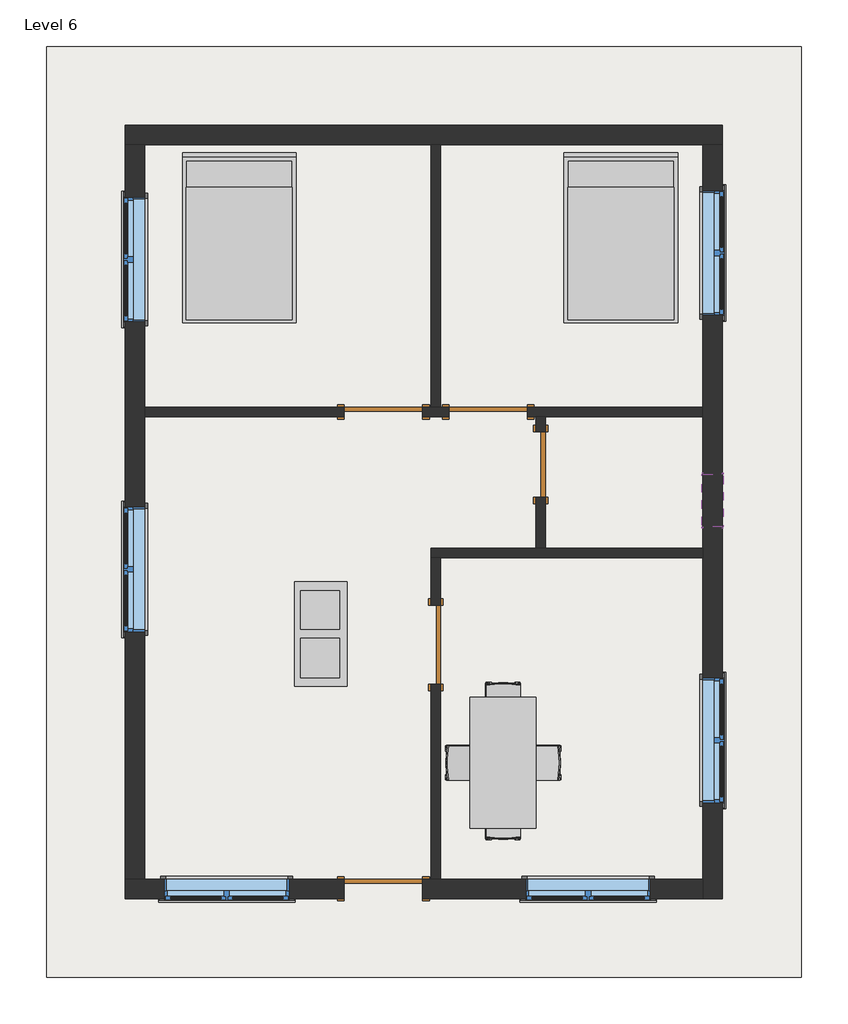
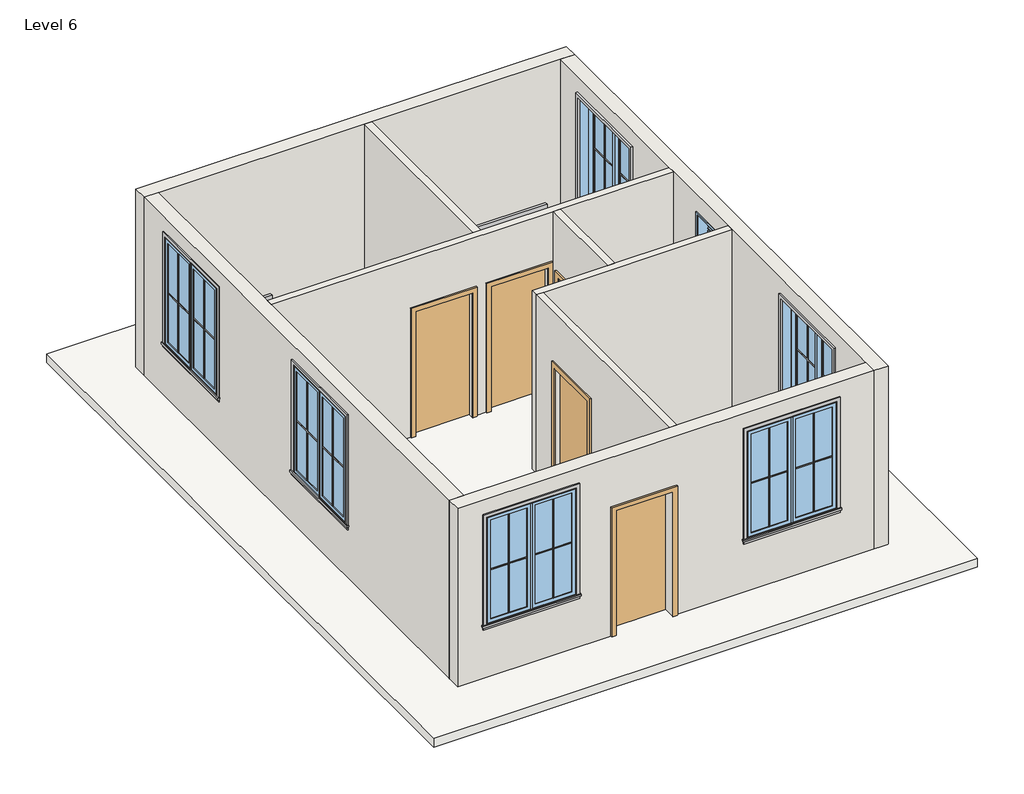
# One storey, incomplete: 25 proxies, 9 walls, 7 windows, 5 doors, 3 furniture elements, 1 roof.
"""IFC4 building model written with IfcOpenShell, lengths in millimetres."""

from ifc_helpers import new_model, si_unit, frame, origin, place, context, project, spatial, polyline, outline, extrude, faceted_brep, transform, mapped, element, save
from components import muntin_pattern_2x2_muntin_pattern_2x2_bff912c5, muntin_pattern_2x2_muntin_pattern_2x2_c2194282, trim_window_exterior_flat_with_sill_e04b3088, trim_window_interior_flat_picture_frame_2a7685fe, coffee_table_with_brass_mullions_11320_coffee_table_with_5962bef7, door_305aa2a5, door_e5f9f3c4, door_0ca8825f, door_f2b275c1, bed_17739_bed_17739_15c61121, dining_table_w_chairs_11374_0cdfc61b, window_9ac97e1a, window_f2d8fef0

model = new_model("IFC4")

# Units and contexts
model_context = context("Model", 3, world=origin())
ifc_project = project(units=[si_unit("LENGTHUNIT", "METRE", prefix="MILLI")], contexts=[model_context])

# Site, building, storey
site = spatial("IfcSite", under=ifc_project)
building = spatial("IfcBuilding", under=site)
storey = spatial("IfcBuildingStorey", under=building, Name="Level 6", Elevation=15849.6)

# Proxies
placement = place(None, origin())
muntin_pattern_2x2_muntin_pattern_2x2_shape = muntin_pattern_2x2_muntin_pattern_2x2_bff912c5(model_context)
element("IfcBuildingElementProxy", 1, Name="Muntin Pattern_2x2 : Muntin Pattern_2x2", ObjectType="Muntin Pattern_2x2 : Muntin Pattern_2x2", at=placement, inside=storey, context=model_context, shape_type="MappedRepresentation", body=[
    mapped(muntin_pattern_2x2_muntin_pattern_2x2_shape, transform((-4718.1437352, -1580.3188735, 16833.85), x_axis=(0.0, 1.0, 0.0), y_axis=(-1.0, 0.0, 0.0), z_axis=(0.0, 0.0, 1.0))),
])
element("IfcBuildingElementProxy", 2, Name="Muntin Pattern_2x2 : Muntin Pattern_2x2", ObjectType="Muntin Pattern_2x2 : Muntin Pattern_2x2", at=placement, inside=storey, context=model_context, shape_type="MappedRepresentation", body=[
    mapped(muntin_pattern_2x2_muntin_pattern_2x2_shape, transform((-3186.2062352, -5039.4813735, 16833.85), x_axis=(-1.0, 0.0, 0.0), y_axis=(0.0, -1.0, 0.0), z_axis=(0.0, 0.0, 1.0))),
])
element("IfcBuildingElementProxy", 3, Name="Muntin Pattern_2x2 : Muntin Pattern_2x2", ObjectType="Muntin Pattern_2x2 : Muntin Pattern_2x2", at=placement, inside=storey, context=model_context, shape_type="MappedRepresentation", body=[
    mapped(muntin_pattern_2x2_muntin_pattern_2x2_shape, transform((1017.4937648, -5039.4813735, 16833.85), x_axis=(-1.0, 0.0, 0.0), y_axis=(0.0, -1.0, 0.0), z_axis=(0.0, 0.0, 1.0))),
])
element("IfcBuildingElementProxy", 4, Name="Muntin Pattern_2x2 : Muntin Pattern_2x2", ObjectType="Muntin Pattern_2x2 : Muntin Pattern_2x2", at=placement, inside=storey, context=model_context, shape_type="MappedRepresentation", body=[
    mapped(muntin_pattern_2x2_muntin_pattern_2x2_shape, transform((2209.7062648, -2847.1438735, 16833.85), x_axis=(0.0, -1.0, 0.0), y_axis=(1.0, 0.0, 0.0), z_axis=(0.0, 0.0, 1.0))),
])
element("IfcBuildingElementProxy", 5, Name="Muntin Pattern_2x2 : Muntin Pattern_2x2", ObjectType="Muntin Pattern_2x2 : Muntin Pattern_2x2", at=placement, inside=storey, context=model_context, shape_type="MappedRepresentation", body=[
    mapped(muntin_pattern_2x2_muntin_pattern_2x2_shape, transform((2209.7062648, 2817.0561265, 16833.85), x_axis=(0.0, -1.0, 0.0), y_axis=(1.0, 0.0, 0.0), z_axis=(0.0, 0.0, 1.0))),
])
element("IfcBuildingElementProxy", 6, Name="Muntin Pattern_2x2 : Muntin Pattern_2x2", ObjectType="Muntin Pattern_2x2 : Muntin Pattern_2x2", at=placement, inside=storey, context=model_context, shape_type="MappedRepresentation", body=[
    mapped(muntin_pattern_2x2_muntin_pattern_2x2_shape, transform((-4718.1437352, 2020.1311265, 16833.85), x_axis=(0.0, 1.0, 0.0), y_axis=(-1.0, 0.0, 0.0), z_axis=(0.0, 0.0, 1.0))),
])
muntin_pattern_2x2_muntin_pattern_2x2_2_shape = muntin_pattern_2x2_muntin_pattern_2x2_c2194282(model_context)
element("IfcBuildingElementProxy", 7, Name="Muntin Pattern_2x2 : Muntin Pattern_2x2", ObjectType="Muntin Pattern_2x2 : Muntin Pattern_2x2", at=placement, inside=storey, context=model_context, shape_type="MappedRepresentation", body=[
    mapped(muntin_pattern_2x2_muntin_pattern_2x2_2_shape, transform((-4718.1437352, -859.5938735, 16833.85), x_axis=(0.0, -1.0, 0.0), y_axis=(1.0, 0.0, 0.0), z_axis=(0.0, 0.0, 1.0))),
])
element("IfcBuildingElementProxy", 8, Name="Muntin Pattern_2x2 : Muntin Pattern_2x2", ObjectType="Muntin Pattern_2x2 : Muntin Pattern_2x2", at=placement, inside=storey, context=model_context, shape_type="MappedRepresentation", body=[
    mapped(muntin_pattern_2x2_muntin_pattern_2x2_2_shape, transform((-3906.9312352, -5039.4813735, 16833.85), x_axis=(1.0, 0.0, 0.0), y_axis=(0.0, 1.0, 0.0), z_axis=(0.0, 0.0, 1.0))),
])
element("IfcBuildingElementProxy", 9, Name="Muntin Pattern_2x2 : Muntin Pattern_2x2", ObjectType="Muntin Pattern_2x2 : Muntin Pattern_2x2", at=placement, inside=storey, context=model_context, shape_type="MappedRepresentation", body=[
    mapped(muntin_pattern_2x2_muntin_pattern_2x2_2_shape, transform((296.7687648, -5039.4813735, 16833.85), x_axis=(1.0, 0.0, 0.0), y_axis=(0.0, 1.0, 0.0), z_axis=(0.0, 0.0, 1.0))),
])
element("IfcBuildingElementProxy", 10, Name="Muntin Pattern_2x2 : Muntin Pattern_2x2", ObjectType="Muntin Pattern_2x2 : Muntin Pattern_2x2", at=placement, inside=storey, context=model_context, shape_type="MappedRepresentation", body=[
    mapped(muntin_pattern_2x2_muntin_pattern_2x2_2_shape, transform((2209.7062648, -3567.8688735, 16833.85), x_axis=(0.0, 1.0, 0.0), y_axis=(-1.0, 0.0, 0.0), z_axis=(0.0, 0.0, 1.0))),
])
element("IfcBuildingElementProxy", 11, Name="Muntin Pattern_2x2 : Muntin Pattern_2x2", ObjectType="Muntin Pattern_2x2 : Muntin Pattern_2x2", at=placement, inside=storey, context=model_context, shape_type="MappedRepresentation", body=[
    mapped(muntin_pattern_2x2_muntin_pattern_2x2_2_shape, transform((2209.7062648, 2096.3311265, 16833.85), x_axis=(0.0, 1.0, 0.0), y_axis=(-1.0, 0.0, 0.0), z_axis=(0.0, 0.0, 1.0))),
])
element("IfcBuildingElementProxy", 12, Name="Muntin Pattern_2x2 : Muntin Pattern_2x2", ObjectType="Muntin Pattern_2x2 : Muntin Pattern_2x2", at=placement, inside=storey, context=model_context, shape_type="MappedRepresentation", body=[
    mapped(muntin_pattern_2x2_muntin_pattern_2x2_2_shape, transform((-4718.1437352, 2740.8561265, 16833.85), x_axis=(0.0, -1.0, 0.0), y_axis=(1.0, 0.0, 0.0), z_axis=(0.0, 0.0, 1.0))),
])
trim_window_exterior_flat_with_sill_shape = trim_window_exterior_flat_with_sill_e04b3088(model_context)
element("IfcBuildingElementProxy", 13, Name="Trim-Window-Exterior-Flat : with Sill", ObjectType="Trim-Window-Exterior-Flat : with Sill", at=placement, inside=storey, context=model_context, shape_type="MappedRepresentation", body=[
    mapped(trim_window_exterior_flat_with_sill_shape, transform((-4727.6687352, -1219.9563735, 18592.8), x_axis=(0.0, -1.0, 0.0), y_axis=(0.0, 0.0, 1.0), z_axis=(-1.0, 0.0, 0.0))),
])
element("IfcBuildingElementProxy", 14, Name="Trim-Window-Exterior-Flat : with Sill", ObjectType="Trim-Window-Exterior-Flat : with Sill", at=placement, inside=storey, context=model_context, shape_type="MappedRepresentation", body=[
    mapped(trim_window_exterior_flat_with_sill_shape, transform((-3546.5687352, -5049.0063735, 18592.8), x_axis=(1.0, 0.0, 0.0), y_axis=(0.0, 0.0, 1.0), z_axis=(0.0, -1.0, 0.0))),
])
element("IfcBuildingElementProxy", 15, Name="Trim-Window-Exterior-Flat : with Sill", ObjectType="Trim-Window-Exterior-Flat : with Sill", at=placement, inside=storey, context=model_context, shape_type="MappedRepresentation", body=[
    mapped(trim_window_exterior_flat_with_sill_shape, transform((657.1312648, -5049.0063735, 18592.8), x_axis=(1.0, 0.0, 0.0), y_axis=(0.0, 0.0, 1.0), z_axis=(0.0, -1.0, 0.0))),
])
element("IfcBuildingElementProxy", 16, Name="Trim-Window-Exterior-Flat : with Sill", ObjectType="Trim-Window-Exterior-Flat : with Sill", at=placement, inside=storey, context=model_context, shape_type="MappedRepresentation", body=[
    mapped(trim_window_exterior_flat_with_sill_shape, transform((2219.2312648, -3207.5063735, 18592.8), x_axis=(0.0, 1.0, 0.0), y_axis=(0.0, 0.0, 1.0), z_axis=(1.0, 0.0, 0.0))),
])
element("IfcBuildingElementProxy", 17, Name="Trim-Window-Exterior-Flat : with Sill", ObjectType="Trim-Window-Exterior-Flat : with Sill", at=placement, inside=storey, context=model_context, shape_type="MappedRepresentation", body=[
    mapped(trim_window_exterior_flat_with_sill_shape, transform((2219.2312648, 2456.6936265, 18592.8), x_axis=(0.0, 1.0, 0.0), y_axis=(0.0, 0.0, 1.0), z_axis=(1.0, 0.0, 0.0))),
])
element("IfcBuildingElementProxy", 18, Name="Trim-Window-Exterior-Flat : with Sill", ObjectType="Trim-Window-Exterior-Flat : with Sill", at=placement, inside=storey, context=model_context, shape_type="MappedRepresentation", body=[
    mapped(trim_window_exterior_flat_with_sill_shape, transform((-4727.6687352, 2380.4936265, 18592.8), x_axis=(0.0, -1.0, 0.0), y_axis=(0.0, 0.0, 1.0), z_axis=(-1.0, 0.0, 0.0))),
])
trim_window_interior_flat_picture_frame_shape = trim_window_interior_flat_picture_frame_2a7685fe(model_context)
element("IfcBuildingElementProxy", 19, Name="Trim-Window-Interior-Flat : Picture Frame", ObjectType="Trim-Window-Interior-Flat : Picture Frame", at=placement, inside=storey, context=model_context, shape_type="MappedRepresentation", body=[
    mapped(trim_window_interior_flat_picture_frame_shape, transform((-4499.0687352, -1219.9563735, 18592.8), x_axis=(0.0, 1.0, 0.0), y_axis=(0.0, 0.0, 1.0), z_axis=(1.0, 0.0, 0.0))),
])
element("IfcBuildingElementProxy", 20, Name="Trim-Window-Interior-Flat : Picture Frame", ObjectType="Trim-Window-Interior-Flat : Picture Frame", at=placement, inside=storey, context=model_context, shape_type="MappedRepresentation", body=[
    mapped(trim_window_interior_flat_picture_frame_shape, transform((-3546.5687352, -4820.4063735, 18592.8), x_axis=(-1.0, 0.0, 0.0), y_axis=(0.0, 0.0, 1.0), z_axis=(0.0, 1.0, 0.0))),
])
element("IfcBuildingElementProxy", 21, Name="Trim-Window-Interior-Flat : Picture Frame", ObjectType="Trim-Window-Interior-Flat : Picture Frame", at=placement, inside=storey, context=model_context, shape_type="MappedRepresentation", body=[
    mapped(trim_window_interior_flat_picture_frame_shape, transform((657.1312648, -4820.4063735, 18592.8), x_axis=(-1.0, 0.0, 0.0), y_axis=(0.0, 0.0, 1.0), z_axis=(0.0, 1.0, 0.0))),
])
element("IfcBuildingElementProxy", 22, Name="Trim-Window-Interior-Flat : Picture Frame", ObjectType="Trim-Window-Interior-Flat : Picture Frame", at=placement, inside=storey, context=model_context, shape_type="MappedRepresentation", body=[
    mapped(trim_window_interior_flat_picture_frame_shape, transform((1990.6312648, -3207.5063735, 18592.8), x_axis=(0.0, -1.0, 0.0), y_axis=(0.0, 0.0, 1.0), z_axis=(-1.0, 0.0, 0.0))),
])
element("IfcBuildingElementProxy", 23, Name="Trim-Window-Interior-Flat : Picture Frame", ObjectType="Trim-Window-Interior-Flat : Picture Frame", at=placement, inside=storey, context=model_context, shape_type="MappedRepresentation", body=[
    mapped(trim_window_interior_flat_picture_frame_shape, transform((1990.6312648, 2456.6936265, 18592.8), x_axis=(0.0, -1.0, 0.0), y_axis=(0.0, 0.0, 1.0), z_axis=(-1.0, 0.0, 0.0))),
])
element("IfcBuildingElementProxy", 24, Name="Trim-Window-Interior-Flat : Picture Frame", ObjectType="Trim-Window-Interior-Flat : Picture Frame", at=placement, inside=storey, context=model_context, shape_type="MappedRepresentation", body=[
    mapped(trim_window_interior_flat_picture_frame_shape, transform((-4499.0687352, 2380.4936265, 18592.8), x_axis=(0.0, 1.0, 0.0), y_axis=(0.0, 0.0, 1.0), z_axis=(1.0, 0.0, 0.0))),
])
coffee_table_with_brass_mullions_11320_coffee_table_with_shape = coffee_table_with_brass_mullions_11320_coffee_table_with_5962bef7(model_context)
element("IfcBuildingElementProxy", 25, Name="coffee_table_with_brass_mullions_11320 : coffee_table_with_brass_mullions_11320", ObjectType="coffee_table_with_brass_mullions_11320 : coffee_table_with_brass_mullions_11320", at=placement, inside=storey, context=model_context, shape_type="MappedRepresentation", body=[
    mapped(coffee_table_with_brass_mullions_11320_coffee_table_with_shape, transform((-2022.5687352, -1334.2563735, 15849.6), x_axis=(0.0, 1.0, 0.0), y_axis=(-1.0, 0.0, 0.0), z_axis=(0.0, 0.0, 1.0))),
])

# Doors
door_shape = door_305aa2a5(model_context)
element("IfcDoor", 26, ObjectType="Single-Flush : 36\" x 84\"", at=placement, inside=storey, context=model_context, shape_type="MappedRepresentation", body=[
    mapped(door_shape, transform((-1114.5187352, -2096.2563735, 15849.6), x_axis=(0.0, 1.0, 0.0), y_axis=(-1.0, 0.0, 0.0), z_axis=(0.0, 0.0, 1.0))),
])
element("IfcDoor", 27, ObjectType="Single-Flush : 36\" x 84\"", at=placement, inside=storey, context=model_context, shape_type="MappedRepresentation", body=[
    mapped(door_shape, transform((-1724.1187352, 608.8436265, 15849.6), x_axis=(-1.0, 0.0, 0.0), y_axis=(0.0, -1.0, 0.0), z_axis=(0.0, 0.0, 1.0))),
])
door_2_shape = door_e5f9f3c4(model_context)
element("IfcDoor", 28, ObjectType="Single-Flush : 36\" x 84\"", at=placement, inside=storey, context=model_context, shape_type="MappedRepresentation", body=[
    mapped(door_2_shape, transform((-504.9187352, 608.8436265, 15849.6), x_axis=(1.0, 0.0, 0.0), y_axis=(0.0, 1.0, 0.0), z_axis=(0.0, 0.0, 1.0))),
])
door_3_shape = door_0ca8825f(model_context)
element("IfcDoor", 29, ObjectType="Single-Flush : 36\" x 84\"", at=placement, inside=storey, context=model_context, shape_type="MappedRepresentation", body=[
    mapped(door_3_shape, transform((-1724.1187352, -4934.7063735, 15849.6), x_axis=(1.0, 0.0, 0.0), y_axis=(0.0, 1.0, 0.0), z_axis=(0.0, 0.0, 1.0))),
])
door_4_shape = door_f2b275c1(model_context)
element("IfcDoor", 30, ObjectType="Single-Flush : DOOR 2'6\"", at=placement, inside=storey, context=model_context, shape_type="MappedRepresentation", body=[
    mapped(door_4_shape, transform((104.6812648, -0.7563735, 15849.6), x_axis=(0.0, 1.0, 0.0), y_axis=(-1.0, 0.0, 0.0), z_axis=(0.0, 0.0, 1.0))),
])

# Furniture
bed_17739_bed_17739_shape = bed_17739_bed_17739_15c61121(model_context)
element("IfcFurniture", 31, ObjectType="Bed_17739 : Bed_17739", at=placement, inside=storey, context=model_context, shape_type="MappedRepresentation", body=[
    mapped(bed_17739_bed_17739_shape, transform((-3400.5187352, 2609.0936265, 15849.6), x_axis=(1.0, 0.0, 0.0), y_axis=(0.0, 1.0, 0.0), z_axis=(0.0, 0.0, 1.0))),
])
element("IfcFurniture", 32, ObjectType="Bed_17739 : Bed_17739", at=placement, inside=storey, context=model_context, shape_type="MappedRepresentation", body=[
    mapped(bed_17739_bed_17739_shape, transform((1038.1312648, 2609.0936265, 15849.6), x_axis=(1.0, 0.0, 0.0), y_axis=(0.0, 1.0, 0.0), z_axis=(0.0, 0.0, 1.0))),
])
dining_table_w_chairs_11374_shape = dining_table_w_chairs_11374_0cdfc61b(model_context)
element("IfcFurniture", 33, ObjectType="Dining_Table_w_Chairs_11374", at=placement, inside=storey, context=model_context, shape_type="MappedRepresentation", body=[
    mapped(dining_table_w_chairs_11374_shape, transform((-238.2576574, -3486.1221401, 15849.6), x_axis=(0.0, 1.0, 0.0), y_axis=(-1.0, 0.0, 0.0), z_axis=(0.0, 0.0, 1.0))),
])

# Roof
element("IfcRoof", 34, ObjectType="ROOF 6\"", at=placement, inside=storey, context=model_context, shape_type="SweptSolid", body=[
    extrude(outline(polyline([(-5642.0687352, 4856.9936265), (3133.6312648, 4856.9936265), (3133.6312648, -5963.4063735), (-5642.0687352, -5963.4063735), (-5642.0687352, 4856.9936265)])), frame((0.0, 0.0, 15697.2), z_axis=(0.0, 0.0, 1.0), x_axis=(1.0, 0.0, 0.0)), (0.0, 0.0, 1.0), 152.4),
])

# Walls
element("IfcWall", 35, ObjectType="WALL 4.5\"", at=placement, inside=storey, context=model_context, shape_type="Brep", body=[
    faceted_brep([(-4499.0687352, 551.6936265, 15849.6), (-2181.3187352, 551.6936265, 15849.6), (-2181.3187352, 551.6936265, 17983.2), (-1266.9187352, 551.6936265, 17983.2), (-1266.9187352, 551.6936265, 15849.6), (-962.1187352, 551.6936265, 15849.6), (-962.1187352, 551.6936265, 17983.2), (-47.7187352, 551.6936265, 17983.2), (-47.7187352, 551.6936265, 15849.6), (47.5312648, 551.6936265, 15849.6), (161.8312648, 551.6936265, 15849.6), (1990.6312648, 551.6936265, 15849.6), (1990.6312648, 551.6936265, 18897.6), (161.8312648, 551.6936265, 18897.6), (47.5312648, 551.6936265, 18897.6), (-4499.0687352, 551.6936265, 18897.6), (-2181.3187352, 665.9936265, 17983.2), (-2181.3187352, 665.9936265, 15849.6), (-4499.0687352, 665.9936265, 15849.6), (-4499.0687352, 665.9936265, 18897.6), (-1171.6687352, 665.9936265, 18897.6), (-1057.3687352, 665.9936265, 18897.6), (1990.6312648, 665.9936265, 18897.6), (1990.6312648, 665.9936265, 15849.6), (-47.7187352, 665.9936265, 15849.6), (-47.7187352, 665.9936265, 17983.2), (-962.1187352, 665.9936265, 17983.2), (-962.1187352, 665.9936265, 15849.6), (-1057.3687352, 665.9936265, 15849.6), (-1171.6687352, 665.9936265, 15849.6), (-1266.9187352, 665.9936265, 15849.6), (-1266.9187352, 665.9936265, 17983.2)], [[[0, 1, 2, 3, 4, 5, 6, 7, 8, 9, 10, 11, 12, 13, 14, 15]], [[16, 17, 18, 19, 20, 21, 22, 23, 24, 25, 26, 27, 28, 29, 30, 31]], [[11, 10, 9, 8, 24, 23]], [[18, 17, 1, 0]], [[30, 29, 28, 27, 5, 4]], [[12, 11, 23, 22]], [[0, 15, 19, 18]], [[25, 24, 8, 7]], [[26, 25, 7, 6]], [[27, 26, 6, 5]], [[2, 1, 17, 16]], [[3, 2, 16, 31]], [[4, 3, 31, 30]], [[15, 14, 13, 12, 22, 21, 20, 19]]]),
])
element("IfcWall", 36, ObjectType="WALL 4.5\"", at=placement, inside=storey, context=model_context, shape_type="SweptSolid", body=[
    extrude(outline(polyline([(-1057.3687352, 3713.9936265), (-1057.3687352, 665.9936265), (-1171.6687352, 665.9936265), (-1171.6687352, 3713.9936265), (-1057.3687352, 3713.9936265)])), frame((0.0, 0.0, 15849.6), z_axis=(0.0, 0.0, 1.0), x_axis=(1.0, 0.0, 0.0)), (0.0, 0.0, 1.0), 3048.0),
])
element("IfcWall", 37, ObjectType="WALL 4.5\"", at=placement, inside=storey, context=model_context, shape_type="Brep", body=[
    faceted_brep([(1990.6312648, -972.3063735, 15849.6), (161.8312648, -972.3063735, 15849.6), (47.5312648, -972.3063735, 15849.6), (-1171.6687352, -972.3063735, 15849.6), (-1171.6687352, -972.3063735, 18897.6), (47.5312648, -972.3063735, 18897.6), (161.8312648, -972.3063735, 18897.6), (1990.6312648, -972.3063735, 18897.6), (1990.6312648, -1086.6063735, 15849.6), (1990.6312648, -1086.6063735, 18897.6), (-1057.3687352, -1086.6063735, 18897.6), (-1171.6687352, -1086.6063735, 18897.6), (-1171.6687352, -1086.6063735, 15849.6), (-1057.3687352, -1086.6063735, 15849.6)], [[[0, 1, 2, 3, 4, 5, 6, 7]], [[8, 9, 10, 11, 12, 13]], [[3, 2, 1, 0, 8, 13, 12]], [[0, 7, 9, 8]], [[4, 3, 12, 11]], [[7, 6, 5, 4, 11, 10, 9]]]),
])
element("IfcWall", 38, ObjectType="WALL 4.5\"", at=placement, inside=storey, context=model_context, shape_type="SweptSolid", body=[
    extrude(outline(polyline([(-1086.6063735, 15849.6), (-1639.0563735, 15849.6), (-1639.0563735, 17983.2), (-2553.4563735, 17983.2), (-2553.4563735, 15849.6), (-4820.4063735, 15849.6), (-4820.4063735, 18897.6), (-1086.6063735, 18897.6), (-1086.6063735, 15849.6)])), frame((-1171.6687352, 0.0, 0.0), z_axis=(1.0, 0.0, 0.0), x_axis=(0.0, 1.0, 0.0)), (0.0, 0.0, 1.0), 114.3),
])
element("IfcWall", 39, ObjectType="WALL 4.5\"", at=placement, inside=storey, context=model_context, shape_type="SweptSolid", body=[
    extrude(outline(polyline([(551.6936265, 15849.6), (380.2436265, 15849.6), (380.2436265, 17881.6), (-381.7563735, 17881.6), (-381.7563735, 15849.6), (-972.3063735, 15849.6), (-972.3063735, 18897.6), (551.6936265, 18897.6), (551.6936265, 15849.6)])), frame((47.5312648, 0.0, 0.0), z_axis=(1.0, 0.0, 0.0), x_axis=(0.0, 1.0, 0.0)), (0.0, 0.0, 1.0), 114.3),
])
element("IfcWall", 40, ObjectType="WALL 9\"", at=placement, inside=storey, context=model_context, shape_type="Brep", body=[
    faceted_brep([(-4727.6687352, 3713.9936265, 15849.6), (-4499.0687352, 3713.9936265, 15849.6), (-1171.6687352, 3713.9936265, 15849.6), (-1057.3687352, 3713.9936265, 15849.6), (1990.6312648, 3713.9936265, 15849.6), (2219.2312648, 3713.9936265, 15849.6), (2219.2312648, 3713.9936265, 18897.6), (1990.6312648, 3713.9936265, 18897.6), (-1057.3687352, 3713.9936265, 18897.6), (-1171.6687352, 3713.9936265, 18897.6), (-4499.0687352, 3713.9936265, 18897.6), (-4727.6687352, 3713.9936265, 18897.6), (-4727.6687352, 3942.5936265, 15849.6), (-4727.6687352, 3942.5936265, 18897.6), (2219.2312648, 3942.5936265, 18897.6), (2219.2312648, 3942.5936265, 15849.6)], [[[0, 1, 2, 3, 4, 5, 6, 7, 8, 9, 10, 11]], [[12, 13, 14, 15]], [[5, 4, 3, 2, 1, 0, 12, 15]], [[6, 5, 15, 14]], [[0, 11, 13, 12]], [[11, 10, 9, 8, 7, 6, 14, 13]]]),
])
element("IfcWall", 41, ObjectType="WALL 9\"", at=placement, inside=storey, context=model_context, shape_type="Brep", body=[
    faceted_brep([(1990.6312648, 3713.9936265, 15849.6), (1990.6312648, 665.9936265, 15849.6), (1990.6312648, 551.6936265, 15849.6), (1990.6312648, -972.3063735, 15849.6), (1990.6312648, -1086.6063735, 15849.6), (1990.6312648, -4820.4063735, 15849.6), (1990.6312648, -5049.0063735, 15849.6), (1990.6312648, -5049.0063735, 18897.6), (1990.6312648, -4820.4063735, 18897.6), (1990.6312648, -1086.6063735, 18897.6), (1990.6312648, -972.3063735, 18897.6), (1990.6312648, 551.6936265, 18897.6), (1990.6312648, 665.9936265, 18897.6), (1990.6312648, 3713.9936265, 18897.6), (1990.6312648, -3931.4063735, 18592.8), (1990.6312648, -3931.4063735, 16764.0), (1990.6312648, -2483.6063735, 16764.0), (1990.6312648, -2483.6063735, 18592.8), (1990.6312648, 1732.7936265, 18592.8), (1990.6312648, 1732.7936265, 16764.0), (1990.6312648, 3180.5936265, 16764.0), (1990.6312648, 3180.5936265, 18592.8), (1990.6312648, -115.0563735, 18592.8), (1990.6312648, -724.6563735, 18592.8), (1990.6312648, -724.6563735, 17983.2), (1990.6312648, -115.0563735, 17983.2), (2219.2312648, 3713.9936265, 15849.6), (2219.2312648, 3713.9936265, 18897.6), (2219.2312648, -5049.0063735, 18897.6), (2219.2312648, -5049.0063735, 15849.6), (2219.2312648, -3931.4063735, 18592.8), (2219.2312648, -2483.6063735, 18592.8), (2219.2312648, -2483.6063735, 16764.0), (2219.2312648, -3931.4063735, 16764.0), (2219.2312648, 1732.7936265, 18592.8), (2219.2312648, 3180.5936265, 18592.8), (2219.2312648, 3180.5936265, 16764.0), (2219.2312648, 1732.7936265, 16764.0), (2219.2312648, -115.0563735, 18592.8), (2219.2312648, -115.0563735, 17983.2), (2219.2312648, -724.6563735, 17983.2), (2219.2312648, -724.6563735, 18592.8)], [[[0, 1, 2, 3, 4, 5, 6, 7, 8, 9, 10, 11, 12, 13], [14, 15, 16, 17], [18, 19, 20, 21], [22, 23, 24, 25]], [[26, 27, 28, 29], [30, 31, 32, 33], [34, 35, 36, 37], [38, 39, 40, 41]], [[6, 5, 4, 3, 2, 1, 0, 26, 29]], [[0, 13, 27, 26]], [[7, 6, 29, 28]], [[15, 14, 30, 33]], [[16, 15, 33, 32]], [[17, 16, 32, 31]], [[14, 17, 31, 30]], [[19, 18, 34, 37]], [[20, 19, 37, 36]], [[21, 20, 36, 35]], [[18, 21, 35, 34]], [[39, 38, 22, 25]], [[40, 39, 25, 24]], [[41, 40, 24, 23]], [[38, 41, 23, 22]], [[13, 12, 11, 10, 9, 8, 7, 28, 27]]]),
])
element("IfcWall", 42, ObjectType="WALL 9\"", at=placement, inside=storey, context=model_context, shape_type="Brep", body=[
    faceted_brep([(1990.6312648, -4820.4063735, 15849.6), (-1057.3687352, -4820.4063735, 15849.6), (-1171.6687352, -4820.4063735, 15849.6), (-1266.9187352, -4820.4063735, 15849.6), (-1266.9187352, -4820.4063735, 17983.2), (-2181.3187352, -4820.4063735, 17983.2), (-2181.3187352, -4820.4063735, 15849.6), (-4499.0687352, -4820.4063735, 15849.6), (-4727.6687352, -4820.4063735, 15849.6), (-4727.6687352, -4820.4063735, 18897.6), (-4499.0687352, -4820.4063735, 18897.6), (-1171.6687352, -4820.4063735, 18897.6), (-1057.3687352, -4820.4063735, 18897.6), (1990.6312648, -4820.4063735, 18897.6), (-4270.4687352, -4820.4063735, 18592.8), (-4270.4687352, -4820.4063735, 16764.0), (-2822.6687352, -4820.4063735, 16764.0), (-2822.6687352, -4820.4063735, 18592.8), (-66.7687352, -4820.4063735, 18592.8), (-66.7687352, -4820.4063735, 16764.0), (1381.0312648, -4820.4063735, 16764.0), (1381.0312648, -4820.4063735, 18592.8), (-1266.9187352, -5049.0063735, 17983.2), (-1266.9187352, -5049.0063735, 15849.6), (1990.6312648, -5049.0063735, 15849.6), (1990.6312648, -5049.0063735, 18897.6), (-4727.6687352, -5049.0063735, 18897.6), (-4727.6687352, -5049.0063735, 15849.6), (-2181.3187352, -5049.0063735, 15849.6), (-2181.3187352, -5049.0063735, 17983.2), (-4270.4687352, -5049.0063735, 18592.8), (-2822.6687352, -5049.0063735, 18592.8), (-2822.6687352, -5049.0063735, 16764.0), (-4270.4687352, -5049.0063735, 16764.0), (-66.7687352, -5049.0063735, 18592.8), (1381.0312648, -5049.0063735, 18592.8), (1381.0312648, -5049.0063735, 16764.0), (-66.7687352, -5049.0063735, 16764.0)], [[[0, 1, 2, 3, 4, 5, 6, 7, 8, 9, 10, 11, 12, 13], [14, 15, 16, 17], [18, 19, 20, 21]], [[22, 23, 24, 25, 26, 27, 28, 29], [30, 31, 32, 33], [34, 35, 36, 37]], [[28, 27, 8, 7, 6]], [[24, 23, 3, 2, 1, 0]], [[0, 13, 25, 24]], [[9, 8, 27, 26]], [[15, 14, 30, 33]], [[16, 15, 33, 32]], [[17, 16, 32, 31]], [[14, 17, 31, 30]], [[19, 18, 34, 37]], [[20, 19, 37, 36]], [[21, 20, 36, 35]], [[18, 21, 35, 34]], [[4, 3, 23, 22]], [[5, 4, 22, 29]], [[6, 5, 29, 28]], [[13, 12, 11, 10, 9, 26, 25]]]),
])
element("IfcWall", 43, ObjectType="WALL 9\"", at=placement, inside=storey, context=model_context, shape_type="Brep", body=[
    faceted_brep([(-4499.0687352, -4820.4063735, 15849.6), (-4499.0687352, 551.6936265, 15849.6), (-4499.0687352, 665.9936265, 15849.6), (-4499.0687352, 3713.9936265, 15849.6), (-4499.0687352, 3713.9936265, 18897.6), (-4499.0687352, 665.9936265, 18897.6), (-4499.0687352, 551.6936265, 18897.6), (-4499.0687352, -4820.4063735, 18897.6), (-4499.0687352, -496.0563735, 18592.8), (-4499.0687352, -496.0563735, 16764.0), (-4499.0687352, -1943.8563735, 16764.0), (-4499.0687352, -1943.8563735, 18592.8), (-4499.0687352, 3104.3936265, 18592.8), (-4499.0687352, 3104.3936265, 16764.0), (-4499.0687352, 1656.5936265, 16764.0), (-4499.0687352, 1656.5936265, 18592.8), (-4727.6687352, -4820.4063735, 15849.6), (-4727.6687352, -4820.4063735, 18897.6), (-4727.6687352, 3713.9936265, 18897.6), (-4727.6687352, 3713.9936265, 15849.6), (-4727.6687352, -496.0563735, 18592.8), (-4727.6687352, -1943.8563735, 18592.8), (-4727.6687352, -1943.8563735, 16764.0), (-4727.6687352, -496.0563735, 16764.0), (-4727.6687352, 3104.3936265, 18592.8), (-4727.6687352, 1656.5936265, 18592.8), (-4727.6687352, 1656.5936265, 16764.0), (-4727.6687352, 3104.3936265, 16764.0)], [[[0, 1, 2, 3, 4, 5, 6, 7], [8, 9, 10, 11], [12, 13, 14, 15]], [[16, 17, 18, 19], [20, 21, 22, 23], [24, 25, 26, 27]], [[3, 2, 1, 0, 16, 19]], [[4, 3, 19, 18]], [[0, 7, 17, 16]], [[9, 8, 20, 23]], [[10, 9, 23, 22]], [[11, 10, 22, 21]], [[8, 11, 21, 20]], [[13, 12, 24, 27]], [[14, 13, 27, 26]], [[15, 14, 26, 25]], [[12, 15, 25, 24]], [[7, 6, 5, 4, 18, 17]]]),
])

# Windows
window_shape = window_9ac97e1a(model_context)
element("IfcWindow", 44, ObjectType="Window-Casement-Double : 57\" x 72\"", at=placement, inside=storey, context=model_context, shape_type="MappedRepresentation", body=[
    mapped(window_shape, transform((-4613.3687352, -1219.9563735, 15849.6), x_axis=(0.0, 1.0, 0.0), y_axis=(-1.0, 0.0, 0.0), z_axis=(0.0, 0.0, 1.0))),
])
element("IfcWindow", 45, ObjectType="Window-Casement-Double : 57\" x 72\"", at=placement, inside=storey, context=model_context, shape_type="MappedRepresentation", body=[
    mapped(window_shape, transform((-3546.5687352, -4934.7063735, 15849.6), x_axis=(-1.0, 0.0, 0.0), y_axis=(0.0, -1.0, 0.0), z_axis=(0.0, 0.0, 1.0))),
])
element("IfcWindow", 46, ObjectType="Window-Casement-Double : 57\" x 72\"", at=placement, inside=storey, context=model_context, shape_type="MappedRepresentation", body=[
    mapped(window_shape, transform((657.1312648, -4934.7063735, 15849.6), x_axis=(-1.0, 0.0, 0.0), y_axis=(0.0, -1.0, 0.0), z_axis=(0.0, 0.0, 1.0))),
])
element("IfcWindow", 47, ObjectType="Window-Casement-Double : 57\" x 72\"", at=placement, inside=storey, context=model_context, shape_type="MappedRepresentation", body=[
    mapped(window_shape, transform((2104.9312648, -3207.5063735, 15849.6), x_axis=(0.0, -1.0, 0.0), y_axis=(1.0, 0.0, 0.0), z_axis=(0.0, 0.0, 1.0))),
])
element("IfcWindow", 48, ObjectType="Window-Casement-Double : 57\" x 72\"", at=placement, inside=storey, context=model_context, shape_type="MappedRepresentation", body=[
    mapped(window_shape, transform((2104.9312648, 2456.6936265, 15849.6), x_axis=(0.0, -1.0, 0.0), y_axis=(1.0, 0.0, 0.0), z_axis=(0.0, 0.0, 1.0))),
])
element("IfcWindow", 49, ObjectType="Window-Casement-Double : 57\" x 72\"", at=placement, inside=storey, context=model_context, shape_type="MappedRepresentation", body=[
    mapped(window_shape, transform((-4613.3687352, 2380.4936265, 15849.6), x_axis=(0.0, 1.0, 0.0), y_axis=(-1.0, 0.0, 0.0), z_axis=(0.0, 0.0, 1.0))),
])
window_2_shape = window_f2d8fef0(model_context)
element("IfcWindow", 50, ObjectType="Window-Louvers : 24\" x 24\"", at=placement, inside=storey, context=model_context, shape_type="MappedRepresentation", body=[
    mapped(window_2_shape, transform((2111.2812648, -419.8563735, 17068.8), x_axis=(0.0, -1.0, 0.0), y_axis=(1.0, 0.0, 0.0), z_axis=(0.0, 0.0, 1.0))),
])

save(model, "model.ifc")

# Revit data of these elements
# Type "Muntin Pattern_2x2 : Muntin Pattern_2x2"
#   Width [instance default] = 4' - 0"
#   Thickness = 0' - 0 1/2"
#   Height [instance default] = 4' - 0"
#   Distance = 0' - 0 3/4"
#   Interior Material [instance default] = none
#   Exterior Material [instance default] = none
#   Default Elevation = 0
# Type "Trim-Window-Exterior-Flat : with Sill"
#   Trim Width = 0' - 2 1/4"
#   Trim Thickness_Picture Frame = 0' - 1 1/4"
#   Trim Thickness_with Sill = 0' - 0 3/4"
#   Sill Thickness = 0' - 1 1/4"
#   Opening Width [instance default] = 2' - 0"
#   Opening Height [instance default] = 3' - 0"
#   Default Elevation = 4' - 0"
#   Sill = yes
#   Picture Frame = no
#   Trim Material [instance default] = none
# Type "Trim-Window-Interior-Flat : Picture Frame"
#   Trim Thickness_Picture Frame = 0' - 1 1/4"
#   Trim Width = 0' - 2 1/4"
#   Trim Thickness_with Sill = 0' - 0 3/4"
#   Sill Thickness = 0' - 1 1/4"
#   Opening Width [instance default] = 2' - 0"
#   Opening Height [instance default] = 3' - 0"
#   Default Elevation = 4' - 0"
#   Sill = no
#   Picture Frame = yes
#   Trim Material [instance default] = none
# Type "coffee_table_with_brass_mullions_11320 : coffee_table_with_brass_mullions_11320"
#   Default Elevation = 0
# Type "Single-Flush : 36\" x 84\""
#   Type Mark = "1"
#   Construction Type Id = "MDOOR"
#   Assembly Code = "C1020"
#   Analytic Construction = "Metal"
#   Thickness = 0' - 2"
#   Heat Transfer Coefficient (U) = 0.651978 BTU/(h·ft²·°F)
#   Height = 7' - 0"
#   Trim Projection Ext = 0' - 1"
#   Trim Projection Int = 0' - 1"
#   Trim Width = 0' - 3"
#   Width = 3' - 0"
#   Define Thermal Properties by = 1
#   Define Thermal Properties by = 1
#   Door Material = Door - Panel
#   Frame Material = Door - Frame
#   Visual Light Transmittance = 0
#   Solar Heat Gain Coefficient = 0
#   Function = (empty or 0)
#   Wall Closure = (empty or 0)
# Type "Single-Flush : DOOR 2'6\""
#   Type Mark = "8"
#   Construction Type Id = "MDOOR"
#   Assembly Code = "C1020"
#   Analytic Construction = "Metal"
#   Thickness = 0' - 2"
#   Heat Transfer Coefficient (U) = 0.651978 BTU/(h·ft²·°F)
#   Height = 6' - 8"
#   Trim Projection Ext = 0' - 1"
#   Trim Projection Int = 0' - 1"
#   Trim Width = 0' - 3"
#   Width = 2' - 6"
#   Define Thermal Properties by = 1
#   Door Material = Door - Panel
#   Frame Material = Door - Frame
#   Visual Light Transmittance = 0
#   Solar Heat Gain Coefficient = 0
#   Function = (empty or 0)
#   Wall Closure = (empty or 0)
# Type "Bed_17739 : Bed_17739"
#   Default Elevation = 0
# Type "Dining_Table_w_Chairs_11374"
#   Default Elevation = 0
#   Assembly Code = ""
# Type "ROOF 6\""
#   Assembly Code = "B1020"
#   Layers, outside or top first: 0' - 6" no material (function 1)
# Type "WALL 4.5\""
#   Assembly Code = "B2010"
#   Layers, outside or top first: 0' - 4 1/2" no material (function 1)
# Type "WALL 9\""
#   Assembly Code = "B2010"
#   Layers, outside or top first: 0' - 9" no material (function 1)
# Type "Window-Casement-Double : 57\" x 72\""
#   Type Mark = "17"
#   Fire Rating = "0.5h"
#   Assembly Code = "B2020100"
#   Analytic Construction = "Double glazing - domestic"
#   Frame Extension [instance default] = 0' - 0 1/4"
#   Window Inset [instance default] = 0' - 0"
#   Wall Thickness [instance default] = 0' - 6"
#   Interior Wall Closure [instance default] = 0' - 2 1/4"
#   Half Width = 2' - 4 1/2"
#   Visual Light Transmittance = 0.81
#   Thermal Resistance (R) = 1.8146 (h·ft²·°F)/BTU
#   Solar Heat Gain Coefficient = 0.76
#   Rough Width = 4' - 9 1/2"
#   Rough Height = 6' - 0 1/2"
#   Height = 6' - 0"
#   Heat Transfer Coefficient (U) = 0.5511 BTU/(h·ft²·°F)
#   Exterior Wall Closure [instance default] = 0' - 1 1/4"
#   Extension Jamb [instance default] = 0' - 2 1/4"
#   Default Sill Height = 3' - 0"
#   Width = 4' - 9"
#   Define Thermal Properties by = 0
#   Muntin Visibility = yes
#   Interior Trim Visibility [instance default] = yes
#   Exterior Trim Visibility [instance default] = yes
#   Extension Jamb Visibility [instance default] = yes
#   Interior Trim Material = Wood - Stained
#   Muntin Pattern = Muntin Pattern_2x2 : Muntin Pattern_2x2
#   Interior Trim = Trim-Window-Interior-Flat : Picture Frame
#   Interior Frame Material = Wood - Stained
#   Glass Panel Material = Glass
#   Exterior Trim Material = Clad - White
#   Exterior Trim = Trim-Window-Exterior-Flat : with Sill
#   Exterior Frame Material = Clad - White
#   Wall Closure = (empty or 0)
# Type "Window-Louvers : 24\" x 24\""
#   Type Mark = "18"
#   Construction Type Id = "GSP4R"
#   Assembly Code = "B20"
#   Analytic Construction = "1/8 in Pilkington single glazing"
#   Visual Light Transmittance = 0.9
#   Thermal Resistance (R) = 1.53941 (h·ft²·°F)/BTU
#   Solar Heat Gain Coefficient = 0.78
#   Max Height = 1' - 11.74264"
#   Height = 2' - 0"
#   Heat Transfer Coefficient (U) = 0.6496 BTU/(h·ft²·°F)
#   Blade Width [instance default] = 1' - 10 1/2"
#   Blade Vertical Thickness = 0' - 0.35355"
#   Blade Thickness = 0' - 0 1/4"
#   Blade Spacing = 0' - 1 1/2"
#   Blade Height = 0' - 1.85355"
#   Blade Depth = 0' - 3"
#   Blade Angle = 45.00°
#   Default Sill Height = 3' - 0"
#   Trim Projection_Exterior = 0' - 0 1/2"
#   Trim Projection_Interior = 0' - 0 1/2"
#   Trim Width_Exterior = 0' - 1 1/2"
#   Trim Width_Interior = 0' - 1 1/2"
#   Width = 2' - 0"
#   Max Blade Count = 12
#   Define Thermal Properties by = 1
#   Blade Count = 12
#   Frame Material = Birch
#   Louver Material = Birch
#   Trim Exterior Material = Birch
#   Trim Interior Material = Birch
#   Wall Closure = (empty or 0)
# Elements 1, 2, 3, 4, 5, 6, 7, 8, 9, 10, 11, 12 (IfcBuildingElementProxy, "Muntin Pattern_2x2 : Muntin Pattern_2x2")
#   Width = 1' - 11 1/8"
#   Height = 5' - 6 1/2"
#   Interior Material = Wood - Stained
#   Exterior Material = Clad - White
#   Phase Created = New Construction
#   Materials on its faces: "Clad - White", "Wood - Stained"
# Elements 13, 14, 15, 16, 17, 18 (IfcBuildingElementProxy, "Trim-Window-Exterior-Flat : with Sill")
#   Opening Width = 4' - 9"
#   Opening Height = 6' - 0"
#   Trim Material = Clad - White
#   Phase Created = New Construction
#   Materials on its faces: "Clad - White"
# Elements 19, 20, 21, 22, 23, 24 (IfcBuildingElementProxy, "Trim-Window-Interior-Flat : Picture Frame")
#   Opening Width = 4' - 9"
#   Opening Height = 6' - 0"
#   Trim Material = Wood - Stained
#   Phase Created = New Construction
#   Materials on its faces: "Wood - Stained"
# Element 25 (IfcBuildingElementProxy, "coffee_table_with_brass_mullions_11320 : coffee_table_with_brass_mullions_11320")
#   Phase Created = New Construction
#   Materials on its faces: "Default Wall", "TABLE", "Glass", "Default"
# Elements 26, 27, 28, 29 (IfcDoor, "Single-Flush : 36\" x 84\"")
#   Phase Created = New Construction
#   Materials on its faces: "Door - Frame", "Door - Panel"
# Element 30 (IfcDoor, "Single-Flush : DOOR 2'6\"")
#   Phase Created = New Construction
#   Materials on its faces: "Door - Frame", "Door - Panel"
# Elements 31, 32 (IfcFurniture, "Bed_17739 : Bed_17739")
#   Phase Created = New Construction
#   Materials on its faces: "legs", "sheets", "bed frame", "Blanket"
# Element 33 (IfcFurniture, "Dining_Table_w_Chairs_11374")
#   Phase Created = New Construction
# Element 34 (IfcRoof, "ROOF 6\"")
#   built-in parameter 1001705 = 52 (stored number, unit not read)
#   built-in parameter 1001701 = -0.5 (stored number, unit not read)
#   built-in parameter 1001710 = 33615
#   Phase Created = New Construction
#   Materials on its faces: "Copper", "Default Roof", "Wood - Stained"
# Elements 35, 36, 37, 38, 39 (IfcWall, "WALL 4.5\"")
#   Top Offset = 0' - 0"
#   Base Offset = 0' - 0"
#   Unconnected Height = 10' - 0"
#   wall height = 10' - 0"
#   Phase Created = New Construction
#   Base Constraint = Level 6
#   Materials on its faces: "Default Wall"
# Elements 40, 41, 42, 43 (IfcWall, "WALL 9\"")
#   Top Offset = 0' - 0"
#   Base Offset = 0' - 0"
#   Unconnected Height = 10' - 0"
#   wall height = 10' - 0"
#   Phase Created = New Construction
#   Base Constraint = Level 6
#   Materials on its faces: "Default Wall", "Parking Stripe"
# Element 44 (IfcWindow, "Window-Casement-Double : 57\" x 72\"")
#   Mark = "36"
#   Window Inset = 0' - 0"
#   Interior Wall Closure = 0' - 2 1/4"
#   Frame Extension = 0' - 0 1/4"
#   Exterior Wall Closure = 0' - 1 1/4"
#   Interior Trim Visibility = yes
#   Exterior Trim Visibility = yes
#   Phase Created = New Construction
#   Materials on its faces: "Wood - Stained", "Glass", "Clad - White"
# Element 45 (IfcWindow, "Window-Casement-Double : 57\" x 72\"")
#   Mark = "37"
#   Window Inset = 0' - 0"
#   Interior Wall Closure = 0' - 2 1/4"
#   Frame Extension = 0' - 0 1/4"
#   Exterior Wall Closure = 0' - 1 1/4"
#   Interior Trim Visibility = yes
#   Exterior Trim Visibility = yes
#   Phase Created = New Construction
#   Materials on its faces: "Wood - Stained", "Glass", "Clad - White"
# Element 46 (IfcWindow, "Window-Casement-Double : 57\" x 72\"")
#   Mark = "38"
#   Window Inset = 0' - 0"
#   Interior Wall Closure = 0' - 2 1/4"
#   Frame Extension = 0' - 0 1/4"
#   Exterior Wall Closure = 0' - 1 1/4"
#   Interior Trim Visibility = yes
#   Exterior Trim Visibility = yes
#   Phase Created = New Construction
#   Materials on its faces: "Wood - Stained", "Glass", "Clad - White"
# Element 47 (IfcWindow, "Window-Casement-Double : 57\" x 72\"")
#   Mark = "39"
#   Window Inset = 0' - 0"
#   Interior Wall Closure = 0' - 2 1/4"
#   Frame Extension = 0' - 0 1/4"
#   Exterior Wall Closure = 0' - 1 1/4"
#   Interior Trim Visibility = yes
#   Exterior Trim Visibility = yes
#   Phase Created = New Construction
#   Materials on its faces: "Wood - Stained", "Glass", "Clad - White"
# Element 48 (IfcWindow, "Window-Casement-Double : 57\" x 72\"")
#   Mark = "40"
#   Window Inset = 0' - 0"
#   Interior Wall Closure = 0' - 2 1/4"
#   Frame Extension = 0' - 0 1/4"
#   Exterior Wall Closure = 0' - 1 1/4"
#   Interior Trim Visibility = yes
#   Exterior Trim Visibility = yes
#   Phase Created = New Construction
#   Materials on its faces: "Wood - Stained", "Glass", "Clad - White"
# Element 49 (IfcWindow, "Window-Casement-Double : 57\" x 72\"")
#   Mark = "41"
#   Window Inset = 0' - 0"
#   Interior Wall Closure = 0' - 2 1/4"
#   Frame Extension = 0' - 0 1/4"
#   Exterior Wall Closure = 0' - 1 1/4"
#   Interior Trim Visibility = yes
#   Exterior Trim Visibility = yes
#   Phase Created = New Construction
#   Materials on its faces: "Wood - Stained", "Glass", "Clad - White"
# Element 50 (IfcWindow, "Window-Louvers : 24\" x 24\"")
#   Mark = "42"
#   Blade Width = 1' - 10 1/2"
#   Phase Created = New Construction
#   Materials on its faces: "Birch"
# Materials
#   "Door - Panel": class "Wood", colour RGB 210 159 95, transparency 0, Cost = 0
#   "Door - Frame": colour RGB 118 70 51, transparency 0, Cost = 0
#   "Wood - Stained": class "Wood", colour RGB 224 178 126, transparency 0, Cost = 0
#   "Glass": class "Glass", colour RGB 0 128 192, transparency 0.75, Description = "Soda Lime Glass", Cost = 0
#   "Clad - White": class "Wood", colour RGB 242 242 238, transparency 0, Cost = 0
#   "Birch": class "Wood", colour RGB 224 178 126, transparency 0, Description = "Betula Alleghaniensis", Cost = 0
#   "Default Wall": colour RGB 128 128 128, transparency 0, Cost = 0
#   "TABLE": class "Generic", colour RGB 120 120 120, transparency 0, Cost = 0
#   "Default": colour RGB 127 127 127, transparency 0, Cost = 0
#   "legs": colour RGB 90 73 37, transparency 0, Cost = 0
#   "sheets": colour RGB 200 195 176, transparency 0, Cost = 0
#   "bed frame": colour RGB 90 73 37, transparency 0, Cost = 0
#   "Blanket": class "System", colour RGB 59 0 1, transparency 0, Cost = 0
#   "Copper": class "Metal", colour RGB 0 0 0, transparency 0, Description = "Copper, matte finish", Cost = 0
#   "Default Roof": colour RGB 88 101 114, transparency 0, Cost = 0
#   "Parking Stripe": class "Paint", colour RGB 250 250 91, transparency 0, Cost = 0
